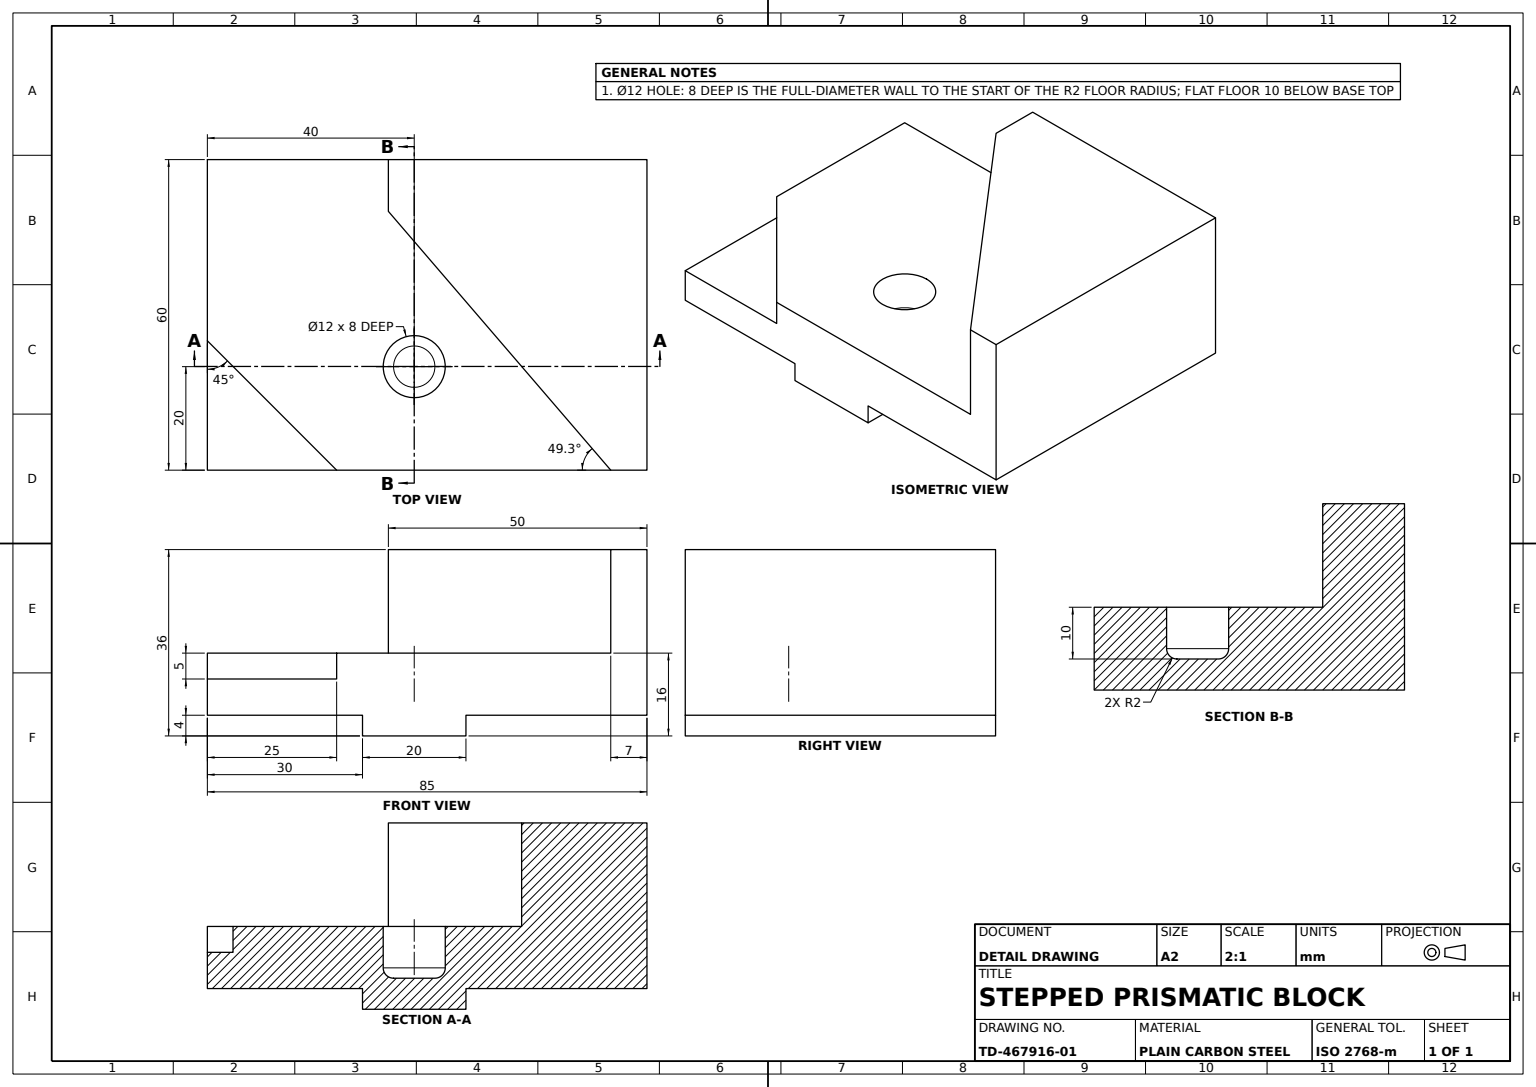
SolidWorks part; units mm, degrees
material "Plain Carbon Steel"
ref_plane "Front Plane" through (0, 0, 0) normal (0, 0, 1) x (1, 0, 0)
ref_plane "Top Plane" through (0, 0, 0) normal (0, 1, 0) x (1, 0, 0)
ref_plane "Right Plane" through (0, 0, 0) normal (1, 0, 0) x (0, 0, -1)
sketch "Base Block Sketch" plane through (0, 0, 0) normal (0, 1, 0) x (1, 0, 0)
  line L1 (-50, 0) -> (35, 0)
  line L2 (-50, 0) -> (-50, 60)
  line L3 (-50, 60) -> (35, 60)
  line L4 (35, 0) -> (35, 60)
  dimension "D1" = 60
  dimension "D2" = 85
  dimension "D3" = 35
extrude "Base Block 85x60x16" add sketch "Base Block Sketch" along normal blind 16
sketch "Underside Step Sketch" plane through (0, 0, 0) normal (0, 0, 1) x (1, 0, 0)
  line L1 (-50, 0) -> (35, 0) construction
  line L2 (0, 0) -> (0, 4)
  line L3 (0, 4) -> (35, 4)
  line L4 (35, 16) -> (35, 0) construction
  line L14 (35, 0) -> (35, 4)
  line L15 (0, 0) -> (35, 0)
  line L16 (-50, 0) -> (-20, 0)
  line L17 (-20, 0) -> (-20, 4)
  line L18 (-20, 4) -> (-50, 4)
  line L19 (-50, 16) -> (-50, 0) construction
  line L20 (-50, 4) -> (-50, 0)
  dimension "D1" = 35
  dimension "D2" = 30
  dimension "D3" = 4
extrude "Underside Step Cut" cut sketch "Underside Step Sketch" against normal through all contours L18 L20 L16 L17
sketch "Relief Cut Sketch" plane through (0, 0, 0) normal (0, 0, 1) x (1, 0, 0)
  line L0 (0, 0) -> (35, 0)
  line L1 (35, 0) -> (35, 4)
  line L2 (35, 16) -> (35, 0) construction
  line L3 (35, 4) -> (0, 4)
  line L4 (0, 4) -> (0, 0)
  dimension "D1" = 4
extrude "Relief Cut 4mm" cut sketch "Relief Cut Sketch" against normal through all
sketch "Raised Block Sketch" plane through (0, 16, 0) normal (0, 1, 0) x (1, 0, 0)
  line L0 (35, 60) -> (-15, 60)
  line L1 (35, 60) -> (-50, 60) construction
  line L2 (-15, 60) -> (-15, 50)
  line L3 (-15, 50) -> (28, 0)
  line L4 (-50, 0) -> (35, 0) construction
  line L5 (28, 0) -> (35, 0)
  line L6 (35, 0) -> (35, 60)
  dimension "D1" = 50
  dimension "D2" = 10
  dimension "D3" = 7
extrude "Raised Block 20mm" add sketch "Raised Block Sketch" along normal blind 20
sketch "Notch Sketch" plane through (0, 16, 0) normal (0, 1, 0) x (1, 0, 0)
  line L0 (-25, 0) -> (-50, 25)
  line L1 (-50, 0) -> (28, 0) construction
  line L2 (-50, 60) -> (-50, 0) construction
  line L3 (-50, 25) -> (-50, 0)
  line L4 (-50, 0) -> (-25, 0)
  dimension "D1" = 25
  dimension "D2" = 25
extrude "Triangular Notch Cut" cut sketch "Notch Sketch" against normal blind 5
sketch "Hole Ø12 Sketch" plane through (0, 16, 0) normal (0, 1, 0) x (1, 0, 0)
  line L2 (-25, 0) -> (28, 0) construction
  line L3 (-50, 60) -> (-50, 25) construction
  circle A0 centre (-10, 20) radius 6
  dimension "D3" = 12
  dimension "D1" = 20
  dimension "D2" = 40
extrude "Hole Ø12x10" cut sketch "Hole Ø12 Sketch" against normal blind 10
fillet "Fillet R2" radius 2 1 edges at (-10, 6, -14)
